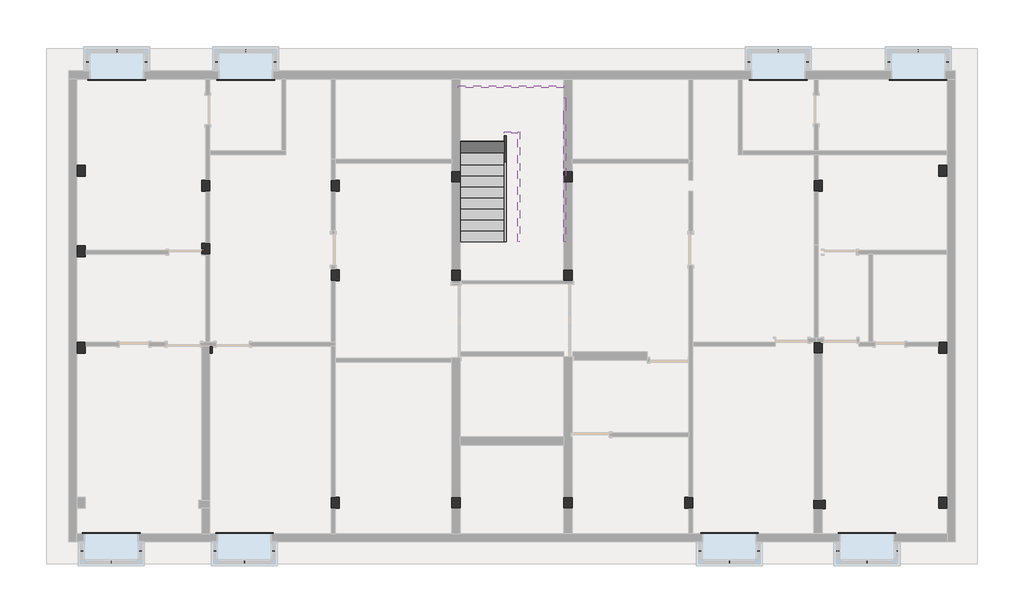
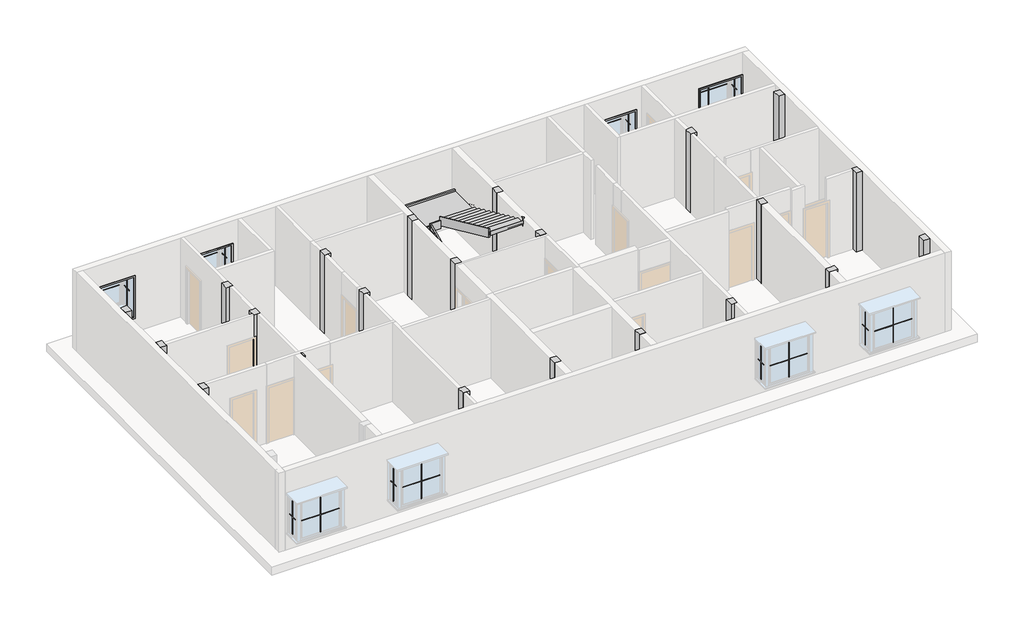
# One storey, part 3 of 3: 32 proxies, 22 columns, 6 members, 1 stair flight.
"""IFC4 building model written with IfcOpenShell, lengths in millimetres."""

from ifc_helpers import new_model, si_unit, frame, origin, place, context, project, spatial, polyline, outline, extrude, faceted_brep, transform, mapped, element, save
from components import m_muntin_pattern_2x2_m_muntin_pattern_2x2_c1fd4460, m_muntin_pattern_2x2_m_muntin_pattern_2x2_777b163a, m_trim_window_interior_flat_picture_frame_44e8afef, stair_flight_7b3ce822

model = new_model("IFC4")

# Units and contexts
model_context = context("Model", 3, world=origin())
ifc_project = project(units=[si_unit("LENGTHUNIT", "METRE", prefix="MILLI")], contexts=[model_context])

# Site, building, storey
site = spatial("IfcSite", under=ifc_project)
building = spatial("IfcBuilding", under=site)
storey = spatial("IfcBuildingStorey", under=building, Elevation=12801.6)

# Proxies
placement = place(None, origin())
m_muntin_pattern_2x2_m_muntin_pattern_2x2_shape = m_muntin_pattern_2x2_m_muntin_pattern_2x2_c1fd4460(model_context)
element("IfcBuildingElementProxy", 1, Name="M_Muntin Pattern_2x2 : M_Muntin Pattern_2x2", ObjectType="M_Muntin Pattern_2x2 : M_Muntin Pattern_2x2", at=placement, inside=storey, context=model_context, shape_type="MappedRepresentation", body=[
    mapped(m_muntin_pattern_2x2_m_muntin_pattern_2x2_shape, transform((-11500.7987957, -5499.9182661, 13522.25), x_axis=(-1.0, 0.0, 0.0), y_axis=(0.0, -1.0, 0.0), z_axis=(0.0, 0.0, 1.0))),
])
element("IfcBuildingElementProxy", 2, Name="M_Muntin Pattern_2x2 : M_Muntin Pattern_2x2", ObjectType="M_Muntin Pattern_2x2 : M_Muntin Pattern_2x2", at=placement, inside=storey, context=model_context, shape_type="MappedRepresentation", body=[
    mapped(m_muntin_pattern_2x2_m_muntin_pattern_2x2_shape, transform((-7819.250543, -5499.9182661, 13522.25), x_axis=(-1.0, 0.0, 0.0), y_axis=(0.0, -1.0, 0.0), z_axis=(0.0, 0.0, 1.0))),
])
element("IfcBuildingElementProxy", 3, Name="M_Muntin Pattern_2x2 : M_Muntin Pattern_2x2", ObjectType="M_Muntin Pattern_2x2 : M_Muntin Pattern_2x2", at=placement, inside=storey, context=model_context, shape_type="MappedRepresentation", body=[
    mapped(m_muntin_pattern_2x2_m_muntin_pattern_2x2_shape, transform((5599.7512082, -5499.9182661, 13522.25), x_axis=(-1.0, 0.0, 0.0), y_axis=(0.0, -1.0, 0.0), z_axis=(0.0, 0.0, 1.0))),
])
element("IfcBuildingElementProxy", 4, Name="M_Muntin Pattern_2x2 : M_Muntin Pattern_2x2", ObjectType="M_Muntin Pattern_2x2 : M_Muntin Pattern_2x2", at=placement, inside=storey, context=model_context, shape_type="MappedRepresentation", body=[
    mapped(m_muntin_pattern_2x2_m_muntin_pattern_2x2_shape, transform((9408.6146942, -5499.9182662, 13522.25), x_axis=(-1.0, 0.0, 0.0), y_axis=(0.0, -1.0, 0.0), z_axis=(0.0, 0.0, 1.0))),
])
element("IfcBuildingElementProxy", 5, Name="M_Muntin Pattern_2x2 : M_Muntin Pattern_2x2", ObjectType="M_Muntin Pattern_2x2 : M_Muntin Pattern_2x2", at=placement, inside=storey, context=model_context, shape_type="MappedRepresentation", body=[
    mapped(m_muntin_pattern_2x2_m_muntin_pattern_2x2_shape, transform((-11348.3987957, 8647.7317329, 13522.25), x_axis=(1.0, 0.0, 0.0), y_axis=(0.0, 1.0, 0.0), z_axis=(0.0, 0.0, 1.0))),
])
element("IfcBuildingElementProxy", 6, Name="M_Muntin Pattern_2x2 : M_Muntin Pattern_2x2", ObjectType="M_Muntin Pattern_2x2 : M_Muntin Pattern_2x2", at=placement, inside=storey, context=model_context, shape_type="MappedRepresentation", body=[
    mapped(m_muntin_pattern_2x2_m_muntin_pattern_2x2_shape, transform((-7779.6987993, 8647.7317329, 13522.25), x_axis=(1.0, 0.0, 0.0), y_axis=(0.0, 1.0, 0.0), z_axis=(0.0, 0.0, 1.0))),
])
element("IfcBuildingElementProxy", 7, Name="M_Muntin Pattern_2x2 : M_Muntin Pattern_2x2", ObjectType="M_Muntin Pattern_2x2 : M_Muntin Pattern_2x2", at=placement, inside=storey, context=model_context, shape_type="MappedRepresentation", body=[
    mapped(m_muntin_pattern_2x2_m_muntin_pattern_2x2_shape, transform((6952.301208, 8647.7317329, 13522.25), x_axis=(1.0, 0.0, 0.0), y_axis=(0.0, 1.0, 0.0), z_axis=(0.0, 0.0, 1.0))),
])
element("IfcBuildingElementProxy", 8, Name="M_Muntin Pattern_2x2 : M_Muntin Pattern_2x2", ObjectType="M_Muntin Pattern_2x2 : M_Muntin Pattern_2x2", at=placement, inside=storey, context=model_context, shape_type="MappedRepresentation", body=[
    mapped(m_muntin_pattern_2x2_m_muntin_pattern_2x2_shape, transform((10825.8012075, 8647.7317329, 13522.25), x_axis=(1.0, 0.0, 0.0), y_axis=(0.0, 1.0, 0.0), z_axis=(0.0, 0.0, 1.0))),
])
m_muntin_pattern_2x2_m_muntin_pattern_2x2_2_shape = m_muntin_pattern_2x2_m_muntin_pattern_2x2_777b163a(model_context)
element("IfcBuildingElementProxy", 9, Name="M_Muntin Pattern_2x2 : M_Muntin Pattern_2x2", ObjectType="M_Muntin Pattern_2x2 : M_Muntin Pattern_2x2", at=placement, inside=storey, context=model_context, shape_type="MappedRepresentation", body=[
    mapped(m_muntin_pattern_2x2_m_muntin_pattern_2x2_2_shape, transform((-10690.4737957, -5190.3932661, 13522.25), x_axis=(0.0, 1.0, 0.0), y_axis=(-1.0, 0.0, 0.0), z_axis=(0.0, 0.0, 1.0))),
])
element("IfcBuildingElementProxy", 10, Name="M_Muntin Pattern_2x2 : M_Muntin Pattern_2x2", ObjectType="M_Muntin Pattern_2x2 : M_Muntin Pattern_2x2", at=placement, inside=storey, context=model_context, shape_type="MappedRepresentation", body=[
    mapped(m_muntin_pattern_2x2_m_muntin_pattern_2x2_2_shape, transform((-12311.1237957, -5190.3932661, 13522.25), x_axis=(0.0, -1.0, 0.0), y_axis=(1.0, 0.0, 0.0), z_axis=(0.0, 0.0, 1.0))),
])
element("IfcBuildingElementProxy", 11, Name="M_Muntin Pattern_2x2 : M_Muntin Pattern_2x2", ObjectType="M_Muntin Pattern_2x2 : M_Muntin Pattern_2x2", at=placement, inside=storey, context=model_context, shape_type="MappedRepresentation", body=[
    mapped(m_muntin_pattern_2x2_m_muntin_pattern_2x2_2_shape, transform((-7008.925543, -5190.3932661, 13522.25), x_axis=(0.0, 1.0, 0.0), y_axis=(-1.0, 0.0, 0.0), z_axis=(0.0, 0.0, 1.0))),
])
element("IfcBuildingElementProxy", 12, Name="M_Muntin Pattern_2x2 : M_Muntin Pattern_2x2", ObjectType="M_Muntin Pattern_2x2 : M_Muntin Pattern_2x2", at=placement, inside=storey, context=model_context, shape_type="MappedRepresentation", body=[
    mapped(m_muntin_pattern_2x2_m_muntin_pattern_2x2_2_shape, transform((-8629.575543, -5190.3932661, 13522.25), x_axis=(0.0, -1.0, 0.0), y_axis=(1.0, 0.0, 0.0), z_axis=(0.0, 0.0, 1.0))),
])
element("IfcBuildingElementProxy", 13, Name="M_Muntin Pattern_2x2 : M_Muntin Pattern_2x2", ObjectType="M_Muntin Pattern_2x2 : M_Muntin Pattern_2x2", at=placement, inside=storey, context=model_context, shape_type="MappedRepresentation", body=[
    mapped(m_muntin_pattern_2x2_m_muntin_pattern_2x2_2_shape, transform((6410.0762082, -5190.3932661, 13522.25), x_axis=(0.0, 1.0, 0.0), y_axis=(-1.0, 0.0, 0.0), z_axis=(0.0, 0.0, 1.0))),
])
element("IfcBuildingElementProxy", 14, Name="M_Muntin Pattern_2x2 : M_Muntin Pattern_2x2", ObjectType="M_Muntin Pattern_2x2 : M_Muntin Pattern_2x2", at=placement, inside=storey, context=model_context, shape_type="MappedRepresentation", body=[
    mapped(m_muntin_pattern_2x2_m_muntin_pattern_2x2_2_shape, transform((4789.4262082, -5190.3932661, 13522.25), x_axis=(0.0, -1.0, 0.0), y_axis=(1.0, 0.0, 0.0), z_axis=(0.0, 0.0, 1.0))),
])
element("IfcBuildingElementProxy", 15, Name="M_Muntin Pattern_2x2 : M_Muntin Pattern_2x2", ObjectType="M_Muntin Pattern_2x2 : M_Muntin Pattern_2x2", at=placement, inside=storey, context=model_context, shape_type="MappedRepresentation", body=[
    mapped(m_muntin_pattern_2x2_m_muntin_pattern_2x2_2_shape, transform((10218.9396942, -5190.3932662, 13522.25), x_axis=(0.0, 1.0, 0.0), y_axis=(-1.0, 0.0, 0.0), z_axis=(0.0, 0.0, 1.0))),
])
element("IfcBuildingElementProxy", 16, Name="M_Muntin Pattern_2x2 : M_Muntin Pattern_2x2", ObjectType="M_Muntin Pattern_2x2 : M_Muntin Pattern_2x2", at=placement, inside=storey, context=model_context, shape_type="MappedRepresentation", body=[
    mapped(m_muntin_pattern_2x2_m_muntin_pattern_2x2_2_shape, transform((8598.2896942, -5190.3932661, 13522.25), x_axis=(0.0, -1.0, 0.0), y_axis=(1.0, 0.0, 0.0), z_axis=(0.0, 0.0, 1.0))),
])
element("IfcBuildingElementProxy", 17, Name="M_Muntin Pattern_2x2 : M_Muntin Pattern_2x2", ObjectType="M_Muntin Pattern_2x2 : M_Muntin Pattern_2x2", at=placement, inside=storey, context=model_context, shape_type="MappedRepresentation", body=[
    mapped(m_muntin_pattern_2x2_m_muntin_pattern_2x2_2_shape, transform((-12158.7237957, 8338.2067329, 13522.25), x_axis=(0.0, -1.0, 0.0), y_axis=(1.0, 0.0, 0.0), z_axis=(0.0, 0.0, 1.0))),
])
element("IfcBuildingElementProxy", 18, Name="M_Muntin Pattern_2x2 : M_Muntin Pattern_2x2", ObjectType="M_Muntin Pattern_2x2 : M_Muntin Pattern_2x2", at=placement, inside=storey, context=model_context, shape_type="MappedRepresentation", body=[
    mapped(m_muntin_pattern_2x2_m_muntin_pattern_2x2_2_shape, transform((-10538.0737957, 8338.2067329, 13522.25), x_axis=(0.0, 1.0, 0.0), y_axis=(-1.0, 0.0, 0.0), z_axis=(0.0, 0.0, 1.0))),
])
element("IfcBuildingElementProxy", 19, Name="M_Muntin Pattern_2x2 : M_Muntin Pattern_2x2", ObjectType="M_Muntin Pattern_2x2 : M_Muntin Pattern_2x2", at=placement, inside=storey, context=model_context, shape_type="MappedRepresentation", body=[
    mapped(m_muntin_pattern_2x2_m_muntin_pattern_2x2_2_shape, transform((-8590.0237993, 8338.2067329, 13522.25), x_axis=(0.0, -1.0, 0.0), y_axis=(1.0, 0.0, 0.0), z_axis=(0.0, 0.0, 1.0))),
])
element("IfcBuildingElementProxy", 20, Name="M_Muntin Pattern_2x2 : M_Muntin Pattern_2x2", ObjectType="M_Muntin Pattern_2x2 : M_Muntin Pattern_2x2", at=placement, inside=storey, context=model_context, shape_type="MappedRepresentation", body=[
    mapped(m_muntin_pattern_2x2_m_muntin_pattern_2x2_2_shape, transform((-6969.3737993, 8338.2067329, 13522.25), x_axis=(0.0, 1.0, 0.0), y_axis=(-1.0, 0.0, 0.0), z_axis=(0.0, 0.0, 1.0))),
])
element("IfcBuildingElementProxy", 21, Name="M_Muntin Pattern_2x2 : M_Muntin Pattern_2x2", ObjectType="M_Muntin Pattern_2x2 : M_Muntin Pattern_2x2", at=placement, inside=storey, context=model_context, shape_type="MappedRepresentation", body=[
    mapped(m_muntin_pattern_2x2_m_muntin_pattern_2x2_2_shape, transform((6141.976208, 8338.2067329, 13522.25), x_axis=(0.0, -1.0, 0.0), y_axis=(1.0, 0.0, 0.0), z_axis=(0.0, 0.0, 1.0))),
])
element("IfcBuildingElementProxy", 22, Name="M_Muntin Pattern_2x2 : M_Muntin Pattern_2x2", ObjectType="M_Muntin Pattern_2x2 : M_Muntin Pattern_2x2", at=placement, inside=storey, context=model_context, shape_type="MappedRepresentation", body=[
    mapped(m_muntin_pattern_2x2_m_muntin_pattern_2x2_2_shape, transform((7762.626208, 8338.2067329, 13522.25), x_axis=(0.0, 1.0, 0.0), y_axis=(-1.0, 0.0, 0.0), z_axis=(0.0, 0.0, 1.0))),
])
element("IfcBuildingElementProxy", 23, Name="M_Muntin Pattern_2x2 : M_Muntin Pattern_2x2", ObjectType="M_Muntin Pattern_2x2 : M_Muntin Pattern_2x2", at=placement, inside=storey, context=model_context, shape_type="MappedRepresentation", body=[
    mapped(m_muntin_pattern_2x2_m_muntin_pattern_2x2_2_shape, transform((10015.4762075, 8338.2067329, 13522.25), x_axis=(0.0, -1.0, 0.0), y_axis=(1.0, 0.0, 0.0), z_axis=(0.0, 0.0, 1.0))),
])
element("IfcBuildingElementProxy", 24, Name="M_Muntin Pattern_2x2 : M_Muntin Pattern_2x2", ObjectType="M_Muntin Pattern_2x2 : M_Muntin Pattern_2x2", at=placement, inside=storey, context=model_context, shape_type="MappedRepresentation", body=[
    mapped(m_muntin_pattern_2x2_m_muntin_pattern_2x2_2_shape, transform((11636.1262075, 8338.2067329, 13522.25), x_axis=(0.0, 1.0, 0.0), y_axis=(-1.0, 0.0, 0.0), z_axis=(0.0, 0.0, 1.0))),
])
m_trim_window_interior_flat_picture_frame_shape = m_trim_window_interior_flat_picture_frame_44e8afef(model_context)
element("IfcBuildingElementProxy", 25, Name="M_Trim-Window-Interior-Flat : Picture Frame", ObjectType="M_Trim-Window-Interior-Flat : Picture Frame", at=placement, inside=storey, context=model_context, shape_type="MappedRepresentation", body=[
    mapped(m_trim_window_interior_flat_picture_frame_shape, transform((-11500.7987957, -4712.5932661, 14952.4), x_axis=(-1.0, 0.0, 0.0), y_axis=(0.0, 0.0, 1.0), z_axis=(0.0, 1.0, 0.0))),
])
element("IfcBuildingElementProxy", 26, Name="M_Trim-Window-Interior-Flat : Picture Frame", ObjectType="M_Trim-Window-Interior-Flat : Picture Frame", at=placement, inside=storey, context=model_context, shape_type="MappedRepresentation", body=[
    mapped(m_trim_window_interior_flat_picture_frame_shape, transform((-7819.250543, -4712.5932661, 14952.4), x_axis=(-1.0, 0.0, 0.0), y_axis=(0.0, 0.0, 1.0), z_axis=(0.0, 1.0, 0.0))),
])
element("IfcBuildingElementProxy", 27, Name="M_Trim-Window-Interior-Flat : Picture Frame", ObjectType="M_Trim-Window-Interior-Flat : Picture Frame", at=placement, inside=storey, context=model_context, shape_type="MappedRepresentation", body=[
    mapped(m_trim_window_interior_flat_picture_frame_shape, transform((5599.7512082, -4712.5932661, 14952.4), x_axis=(-1.0, 0.0, 0.0), y_axis=(0.0, 0.0, 1.0), z_axis=(0.0, 1.0, 0.0))),
])
element("IfcBuildingElementProxy", 28, Name="M_Trim-Window-Interior-Flat : Picture Frame", ObjectType="M_Trim-Window-Interior-Flat : Picture Frame", at=placement, inside=storey, context=model_context, shape_type="MappedRepresentation", body=[
    mapped(m_trim_window_interior_flat_picture_frame_shape, transform((9408.6146942, -4712.5932661, 14952.4), x_axis=(-1.0, 0.0, 0.0), y_axis=(0.0, 0.0, 1.0), z_axis=(0.0, 1.0, 0.0))),
])
element("IfcBuildingElementProxy", 29, Name="M_Trim-Window-Interior-Flat : Picture Frame", ObjectType="M_Trim-Window-Interior-Flat : Picture Frame", at=placement, inside=storey, context=model_context, shape_type="MappedRepresentation", body=[
    mapped(m_trim_window_interior_flat_picture_frame_shape, transform((-11348.3987957, 7860.4067329, 14952.4), x_axis=(1.0, 0.0, 0.0), y_axis=(0.0, 0.0, 1.0), z_axis=(0.0, -1.0, 0.0))),
])
element("IfcBuildingElementProxy", 30, Name="M_Trim-Window-Interior-Flat : Picture Frame", ObjectType="M_Trim-Window-Interior-Flat : Picture Frame", at=placement, inside=storey, context=model_context, shape_type="MappedRepresentation", body=[
    mapped(m_trim_window_interior_flat_picture_frame_shape, transform((-7779.6987993, 7860.4067329, 14952.4), x_axis=(1.0, 0.0, 0.0), y_axis=(0.0, 0.0, 1.0), z_axis=(0.0, -1.0, 0.0))),
])
element("IfcBuildingElementProxy", 31, Name="M_Trim-Window-Interior-Flat : Picture Frame", ObjectType="M_Trim-Window-Interior-Flat : Picture Frame", at=placement, inside=storey, context=model_context, shape_type="MappedRepresentation", body=[
    mapped(m_trim_window_interior_flat_picture_frame_shape, transform((6952.301208, 7860.4067329, 14952.4), x_axis=(1.0, 0.0, 0.0), y_axis=(0.0, 0.0, 1.0), z_axis=(0.0, -1.0, 0.0))),
])
element("IfcBuildingElementProxy", 32, Name="M_Trim-Window-Interior-Flat : Picture Frame", ObjectType="M_Trim-Window-Interior-Flat : Picture Frame", at=placement, inside=storey, context=model_context, shape_type="MappedRepresentation", body=[
    mapped(m_trim_window_interior_flat_picture_frame_shape, transform((10825.8012075, 7860.4067329, 14952.4), x_axis=(1.0, 0.0, 0.0), y_axis=(0.0, 0.0, 1.0), z_axis=(0.0, -1.0, 0.0))),
])

# Columns
element("IfcColumn", 33, ObjectType="Rectangular Column : 1'X 9\"", at=placement, inside=storey, context=model_context, shape_type="SweptSolid", body=[
    extrude(outline(polyline([(-12224.6987957, 583.3067334), (-12224.6987957, 278.5067334), (-12453.2987957, 278.5067334), (-12453.2987957, 583.3067334), (-12224.6987957, 583.3067334)])), frame((0.0, 0.0, 12801.6), z_axis=(0.0, 0.0, 1.0), x_axis=(1.0, 0.0, 0.0)), (0.0, 0.0, 1.0), 3048.0),
])
element("IfcColumn", 34, ObjectType="Rectangular Column : 1'X 9\"", at=placement, inside=storey, context=model_context, shape_type="SweptSolid", body=[
    extrude(outline(polyline([(-12224.6987957, 3256.6567332), (-12224.6987957, 2951.8567332), (-12453.2987957, 2951.8567332), (-12453.2987957, 3256.6567332), (-12224.6987957, 3256.6567332)])), frame((0.0, 0.0, 12801.6), z_axis=(0.0, 0.0, 1.0), x_axis=(1.0, 0.0, 0.0)), (0.0, 0.0, 1.0), 3048.0),
])
element("IfcColumn", 35, ObjectType="Rectangular Column : 1'X 9\"", at=placement, inside=storey, context=model_context, shape_type="Brep", body=[
    faceted_brep([(-8770.2987992, 5066.406733, 12801.6), (-8770.2987992, 4761.606733, 12801.6), (-8884.5987992, 4761.606733, 12801.6), (-8998.8987992, 4761.606733, 12801.6), (-8998.8987992, 5066.406733, 12801.6), (-8884.5987992, 5066.406733, 12801.6), (-8770.2987992, 5066.406733, 15849.6), (-8770.2987992, 4761.606733, 15849.6), (-8884.5987992, 4761.606733, 15849.6), (-8998.8987992, 4761.606733, 15849.6), (-8998.8987992, 5066.406733, 15849.6), (-8884.5987992, 5066.406733, 15849.6)], [[[0, 1, 2, 3, 4, 5]], [[6, 7, 1, 0]], [[7, 8, 9, 3, 2, 1]], [[9, 10, 4, 3]], [[10, 11, 6, 0, 5, 4]], [[6, 11, 10, 9, 8, 7]]]),
])
element("IfcColumn", 36, ObjectType="Rectangular Column : 1'X 9\"", at=placement, inside=storey, context=model_context, shape_type="Brep", body=[
    faceted_brep([(-8770.2987992, 3326.5067332, 12801.6), (-8770.2987992, 3021.7067332, 12801.6), (-8884.598796, 3021.7067332, 12801.6), (-8998.8987992, 3021.7067332, 12801.6), (-8998.8987992, 3326.5067332, 12801.6), (-8884.5987992, 3326.5067332, 12801.6), (-8770.2987992, 3326.5067332, 15849.6), (-8770.2987992, 3021.7067332, 15849.6), (-8884.598796, 3021.7067332, 15849.6), (-8998.8987992, 3021.7067332, 15849.6), (-8998.8987992, 3326.5067332, 15849.6), (-8884.5987992, 3326.5067332, 15849.6)], [[[0, 1, 2, 3, 4, 5]], [[6, 7, 1, 0]], [[7, 8, 9, 3, 2, 1]], [[9, 10, 4, 3]], [[10, 11, 6, 0, 5, 4]], [[6, 11, 10, 9, 8, 7]]]),
])
element("IfcColumn", 37, ObjectType="Rectangular Column : 1'X 9\"", at=placement, inside=storey, context=model_context, shape_type="SweptSolid", body=[
    extrude(outline(polyline([(-8713.148796, 278.5067334), (-8771.750543, 278.5067334), (-8771.750543, 469.0067334), (-8713.148796, 469.0067334), (-8713.148796, 278.5067334)])), frame((0.0, 0.0, 12801.6), z_axis=(0.0, 0.0, 1.0), x_axis=(1.0, 0.0, 0.0)), (0.0, 0.0, 1.0), 3048.0),
])
element("IfcColumn", 38, ObjectType="Rectangular Column : 1'X 9\"", at=placement, inside=storey, context=model_context, shape_type="Brep", body=[
    faceted_brep([(-5188.8987995, 5066.406733, 12801.6), (-5188.8987995, 4761.606733, 12801.6), (-5303.1987995, 4761.606733, 12801.6), (-5417.4987995, 4761.606733, 12801.6), (-5417.4987995, 5066.406733, 12801.6), (-5303.1987995, 5066.406733, 12801.6), (-5188.8987995, 5066.406733, 15849.6), (-5188.8987995, 4761.606733, 15849.6), (-5303.1987995, 4761.606733, 15849.6), (-5417.4987995, 4761.606733, 15849.6), (-5417.4987995, 5066.406733, 15849.6), (-5303.1987995, 5066.406733, 15849.6)], [[[0, 1, 2, 3, 4, 5]], [[6, 7, 1, 0]], [[7, 8, 9, 3, 2, 1]], [[9, 10, 4, 3]], [[10, 11, 6, 0, 5, 4]], [[6, 11, 10, 9, 8, 7]]]),
])
element("IfcColumn", 39, ObjectType="Rectangular Column : 1'X 9\"", at=placement, inside=storey, context=model_context, shape_type="Brep", body=[
    faceted_brep([(-5188.8987995, 2589.9067802, 12801.6), (-5188.8987995, 2285.1067802, 12801.6), (-5303.1987995, 2285.1067802, 12801.6), (-5417.4987995, 2285.1067802, 12801.6), (-5417.4987995, 2589.9067802, 12801.6), (-5303.1987995, 2589.9067802, 12801.6), (-5188.8987995, 2589.9067802, 15849.6), (-5188.8987995, 2285.1067802, 15849.6), (-5303.1987995, 2285.1067802, 15849.6), (-5417.4987995, 2285.1067802, 15849.6), (-5417.4987995, 2589.9067802, 15849.6), (-5303.1987995, 2589.9067802, 15849.6)], [[[0, 1, 2, 3, 4, 5]], [[6, 7, 1, 0]], [[7, 8, 9, 3, 2, 1]], [[9, 10, 4, 3]], [[10, 11, 6, 0, 5, 4]], [[6, 11, 10, 9, 8, 7]]]),
])
element("IfcColumn", 40, ObjectType="Rectangular Column : 1'X 9\"", at=placement, inside=storey, context=model_context, shape_type="Brep", body=[
    faceted_brep([(-5188.8987963, -3709.2932193, 12801.6), (-5188.8987963, -4014.0932193, 12801.6), (-5303.1987963, -4014.0932193, 12801.6), (-5417.4987963, -4014.0932193, 12801.6), (-5417.4987963, -3709.2932193, 12801.6), (-5303.1987995, -3709.2932193, 12801.6), (-5188.8987963, -3709.2932193, 15849.6), (-5188.8987963, -4014.0932193, 15849.6), (-5303.1987963, -4014.0932193, 15849.6), (-5417.4987963, -4014.0932193, 15849.6), (-5417.4987963, -3709.2932193, 15849.6), (-5303.1987995, -3709.2932193, 15849.6)], [[[0, 1, 2, 3, 4, 5]], [[6, 7, 1, 0]], [[7, 8, 9, 3, 2, 1]], [[9, 10, 4, 3]], [[10, 11, 6, 0, 5, 4]], [[6, 11, 10, 9, 8, 7]]]),
])
element("IfcColumn", 41, ObjectType="Rectangular Column : 1'X 9\"", at=placement, inside=storey, context=model_context, shape_type="SweptSolid", body=[
    extrude(outline(polyline([(1250.0012085, -3709.2932193), (1250.0012085, -4014.0932193), (1021.4012085, -4014.0932193), (1021.4012085, -3709.2932193), (1250.0012085, -3709.2932193)])), frame((0.0, 0.0, 12801.6), z_axis=(0.0, 0.0, 1.0), x_axis=(1.0, 0.0, 0.0)), (0.0, 0.0, 1.0), 3048.0),
])
element("IfcColumn", 42, ObjectType="Rectangular Column : 1'X 9\"", at=placement, inside=storey, context=model_context, shape_type="Brep", body=[
    faceted_brep([(4590.1012082, -3709.2932193, 12801.6), (4590.1012082, -4014.0932193, 12801.6), (4475.8012082, -4014.0932193, 12801.6), (4361.5012082, -4014.0932193, 12801.6), (4361.5012082, -3709.2932193, 12801.6), (4475.8012082, -3709.2932193, 12801.6), (4590.1012082, -3709.2932193, 15849.6), (4590.1012082, -4014.0932193, 15849.6), (4475.8012082, -4014.0932193, 15849.6), (4361.5012082, -4014.0932193, 15849.6), (4361.5012082, -3709.2932193, 15849.6), (4475.8012082, -3709.2932193, 15849.6)], [[[0, 1, 2, 3, 4, 5]], [[6, 7, 1, 0]], [[7, 8, 9, 3, 2, 1]], [[9, 10, 4, 3]], [[10, 11, 6, 0, 5, 4]], [[6, 11, 10, 9, 8, 7]]]),
])
element("IfcColumn", 43, ObjectType="Rectangular Column : 1'X 9\"", at=placement, inside=storey, context=model_context, shape_type="SweptSolid", body=[
    extrude(outline(polyline([(11625.9012075, -3709.2932671), (11625.9012075, -4014.0932671), (11397.3012075, -4014.0932671), (11397.3012075, -3709.2932671), (11625.9012075, -3709.2932671)])), frame((0.0, 0.0, 12801.6), z_axis=(0.0, 0.0, 1.0), x_axis=(1.0, 0.0, 0.0)), (0.0, 0.0, 1.0), 3048.0),
])
element("IfcColumn", 44, ObjectType="Rectangular Column : 1'X 9\"", at=placement, inside=storey, context=model_context, shape_type="Brep", body=[
    faceted_brep([(11625.9012075, 583.3067295, 12801.6), (11625.9012075, 278.5067295, 12801.6), (11397.3012075, 278.5067295, 12801.6), (11397.3012075, 469.0067295, 12801.6), (11397.3012075, 583.3067295, 12801.6), (11625.9012075, 583.3067295, 15849.6), (11625.9012075, 278.5067295, 15849.6), (11397.3012075, 278.5067295, 15849.6), (11397.3012075, 469.0067295, 15849.6), (11397.3012075, 583.3067295, 15849.6)], [[[0, 1, 2, 3, 4]], [[5, 6, 1, 0]], [[6, 7, 2, 1]], [[7, 8, 9, 4, 3, 2]], [[9, 5, 0, 4]], [[5, 9, 8, 7, 6]]]),
])
element("IfcColumn", 45, ObjectType="Rectangular Column : 1'X 9\"", at=placement, inside=storey, context=model_context, shape_type="SweptSolid", body=[
    extrude(outline(polyline([(11625.9012075, 5479.1567329), (11625.9012075, 5174.3567329), (11397.3012075, 5174.3567329), (11397.3012075, 5479.1567329), (11625.9012075, 5479.1567329)])), frame((0.0, 0.0, 12801.6), z_axis=(0.0, 0.0, 1.0), x_axis=(1.0, 0.0, 0.0)), (0.0, 0.0, 1.0), 3048.0),
])
element("IfcColumn", 46, ObjectType="Rectangular Column : 1'X 9\"", at=placement, inside=storey, context=model_context, shape_type="Brep", body=[
    faceted_brep([(8172.5040565, 5065.4824989, 12801.6), (8172.5040565, 4760.6824989, 12801.6), (8057.2012047, 4760.6824989, 12801.6), (7943.9040565, 4760.6824989, 12801.6), (7943.9040565, 5065.4824989, 12801.6), (8058.2040565, 5065.4824989, 12801.6), (8172.5040565, 5065.4824989, 15849.6), (8172.5040565, 4760.6824989, 15849.6), (8057.2012047, 4760.6824989, 15849.6), (7943.9040565, 4760.6824989, 15849.6), (7943.9040565, 5065.4824989, 15849.6), (8058.2040565, 5065.4824989, 15849.6)], [[[0, 1, 2, 3, 4, 5]], [[6, 7, 1, 0]], [[7, 8, 9, 3, 2, 1]], [[9, 10, 4, 3]], [[10, 11, 6, 0, 5, 4]], [[6, 11, 10, 9, 8, 7]]]),
])
element("IfcColumn", 47, ObjectType="Rectangular Column : 1'X 9\"", at=placement, inside=storey, context=model_context, shape_type="Brep", body=[
    faceted_brep([(8171.5012047, 583.3067334, 12801.6), (8171.5012047, 278.5067334, 12801.6), (7942.9012047, 278.5067334, 12801.6), (7942.9012047, 583.3067334, 12801.6), (8000.0512079, 583.3067334, 12801.6), (8171.5012047, 583.3067334, 15849.6), (8171.5012047, 278.5067334, 15849.6), (7942.9012047, 278.5067334, 15849.6), (7942.9012047, 583.3067334, 15849.6), (8000.0512079, 583.3067334, 15849.6)], [[[0, 1, 2, 3, 4]], [[5, 6, 1, 0]], [[6, 7, 2, 1]], [[7, 8, 3, 2]], [[8, 9, 5, 0, 4, 3]], [[5, 9, 8, 7, 6]]]),
])
element("IfcColumn", 48, ObjectType="Rectangular Column : 1'X 9\"", at=placement, inside=storey, context=model_context, shape_type="Brep", body=[
    faceted_brep([(7941.7646942, -3787.3914801, 12801.6), (8246.5646942, -3787.3914801, 12801.6), (8246.5646942, -4015.9914801, 12801.6), (8170.3646942, -4015.9914801, 12801.6), (7941.7646942, -4015.9914801, 12801.6), (7941.7646942, -3787.3914801, 15849.6), (8246.5646942, -3787.3914801, 15849.6), (8246.5646942, -4015.9914801, 15849.6), (8170.3646942, -4015.9914801, 15849.6), (7941.7646942, -4015.9914801, 15849.6)], [[[0, 1, 2, 3, 4]], [[5, 6, 1, 0]], [[6, 7, 2, 1]], [[7, 8, 9, 4, 3, 2]], [[9, 5, 0, 4]], [[5, 9, 8, 7, 6]]]),
])
element("IfcColumn", 49, ObjectType="Rectangular Column : 1'X 9\"", at=placement, inside=storey, context=model_context, shape_type="SweptSolid", body=[
    extrude(outline(polyline([(-12453.2987957, 5174.3567339), (-12453.2987957, 5479.1567339), (-12224.6987957, 5479.1567339), (-12224.6987957, 5174.3567339), (-12453.2987957, 5174.3567339)])), frame((0.0, 0.0, 12801.6), z_axis=(0.0, 0.0, 1.0), x_axis=(1.0, 0.0, 0.0)), (0.0, 0.0, 1.0), 3048.0),
])
element("IfcColumn", 50, ObjectType="Rectangular Column : 1'X 9\"", at=placement, inside=storey, context=model_context, shape_type="SweptSolid", body=[
    extrude(outline(polyline([(-1845.5417538, 5320.4067329), (-1845.5417538, 5015.6067329), (-2074.1417538, 5015.6067329), (-2074.1417538, 5320.4067329), (-1845.5417538, 5320.4067329)])), frame((0.0, 0.0, 12801.6), z_axis=(0.0, 0.0, 1.0), x_axis=(1.0, 0.0, 0.0)), (0.0, 0.0, 1.0), 3048.0),
])
element("IfcColumn", 51, ObjectType="Rectangular Column : 1'X 9\"", at=placement, inside=storey, context=model_context, shape_type="SweptSolid", body=[
    extrude(outline(polyline([(1250.0012085, 5320.4067329), (1250.0012085, 5015.6067329), (1021.4012085, 5015.6067329), (1021.4012085, 5320.4067329), (1250.0012085, 5320.4067329)])), frame((0.0, 0.0, 12801.6), z_axis=(0.0, 0.0, 1.0), x_axis=(1.0, 0.0, 0.0)), (0.0, 0.0, 1.0), 3048.0),
])
element("IfcColumn", 52, ObjectType="Rectangular Column : 1'X 9\"", at=placement, inside=storey, context=model_context, shape_type="SweptSolid", body=[
    extrude(outline(polyline([(-1845.5417538, 2589.906774), (-1845.5417538, 2285.106774), (-2074.1417538, 2285.106774), (-2074.1417538, 2589.906774), (-1845.5417538, 2589.906774)])), frame((0.0, 0.0, 12801.6), z_axis=(0.0, 0.0, 1.0), x_axis=(1.0, 0.0, 0.0)), (0.0, 0.0, 1.0), 3048.0),
])
element("IfcColumn", 53, ObjectType="Rectangular Column : 1'X 9\"", at=placement, inside=storey, context=model_context, shape_type="Brep", body=[
    faceted_brep([(1253.2582462, 2589.9067742, 12801.6), (1253.2582462, 2285.1067742, 12801.6), (1024.6582462, 2285.1067742, 12801.6), (1024.6582462, 2589.9067742, 12801.6), (1250.0012085, 2589.9067742, 12801.6), (1253.2582462, 2589.9067742, 15849.6), (1253.2582462, 2285.1067742, 15849.6), (1024.6582462, 2285.1067742, 15849.6), (1024.6582462, 2589.9067742, 15849.6), (1250.0012085, 2589.9067742, 15849.6)], [[[0, 1, 2, 3, 4]], [[5, 6, 1, 0]], [[6, 7, 2, 1]], [[7, 8, 3, 2]], [[8, 9, 5, 0, 4, 3]], [[5, 9, 8, 7, 6]]]),
])
element("IfcColumn", 54, ObjectType="Rectangular Column : 1'X 9\"", at=placement, inside=storey, context=model_context, shape_type="SweptSolid", body=[
    extrude(outline(polyline([(-1848.7987998, -3709.2932663), (-1848.7987998, -4014.0932663), (-2077.3987998, -4014.0932663), (-2077.3987998, -3709.2932663), (-1848.7987998, -3709.2932663)])), frame((0.0, 0.0, 12801.6), z_axis=(0.0, 0.0, 1.0), x_axis=(1.0, 0.0, 0.0)), (0.0, 0.0, 1.0), 3048.0),
])

# Members
element("IfcMember", 55, ObjectType="Stringer - 2\" Width", at=placement, inside=storey, context=model_context, shape_type="SweptSolid", body=[
    extrude(outline(polyline([(3364.6067329, 12801.6), (3364.6067329, 13001.4262721), (6445.4289342, 14401.8), (7182.0114168, 14401.8), (3661.5714168, 12801.6), (3364.6067329, 12801.6)])), frame((-1896.3417538, 0.0, 0.0), z_axis=(1.0, 0.0, 0.0), x_axis=(0.0, 1.0, 0.0)), (0.0, 0.0, 1.0), 50.8),
])
element("IfcMember", 56, ObjectType="Stringer - 2\" Width", at=placement, inside=storey, context=model_context, shape_type="SweptSolid", body=[
    extrude(outline(polyline([(-1896.3417538, 7631.8067329), (-1896.3417538, 7682.6067329), (1021.4012085, 7682.6067329), (1021.4012085, 7631.8067329), (-1896.3417538, 7631.8067329)])), frame((0.0, 0.0, 14097.0), z_axis=(0.0, 0.0, 1.0), x_axis=(1.0, 0.0, 0.0)), (0.0, 0.0, 1.0), 304.8),
])
element("IfcMember", 57, ObjectType="Stringer - 2\" Width", at=placement, inside=storey, context=model_context, shape_type="SweptSolid", body=[
    extrude(outline(polyline([(6618.562049, 14097.0), (3364.6067329, 15576.0705982), (3364.6067329, 15910.8808176), (7355.1445316, 14097.0), (6618.562049, 14097.0)])), frame((1021.4012085, 0.0, 0.0), z_axis=(1.0, 0.0, 0.0), x_axis=(0.0, 1.0, 0.0)), (0.0, 0.0, 1.0), 50.8),
])
element("IfcMember", 58, ObjectType="Stringer - 2\" Width", at=placement, inside=storey, context=model_context, shape_type="SweptSolid", body=[
    extrude(outline(polyline([(3364.6067329, 12801.6), (3364.6067329, 13001.4262721), (6361.8067329, 14363.7899085), (6361.8067329, 14028.9796892), (3661.5714168, 12801.6), (3364.6067329, 12801.6)])), frame((-629.5987998, 0.0, 0.0), z_axis=(1.0, 0.0, 0.0), x_axis=(0.0, 1.0, 0.0)), (0.0, 0.0, 1.0), 50.8),
])
element("IfcMember", 59, ObjectType="Stringer - 2\" Width", at=placement, inside=storey, context=model_context, shape_type="SweptSolid", body=[
    extrude(outline(polyline([(-629.5987998, 6361.8067329), (-629.5987998, 6412.6067329), (-248.5987915, 6412.6067329), (-248.5987915, 6361.8067329), (-629.5987998, 6361.8067329)])), frame((0.0, 0.0, 14097.0), z_axis=(0.0, 0.0, 1.0), x_axis=(1.0, 0.0, 0.0)), (0.0, 0.0, 1.0), 304.8),
])
element("IfcMember", 60, ObjectType="Stringer - 2\" Width", at=placement, inside=storey, context=model_context, shape_type="SweptSolid", body=[
    extrude(outline(polyline([(6412.6067329, 14525.4262721), (6412.6067329, 14190.6160528), (3364.6067329, 15576.0705982), (3364.6067329, 15910.8808176), (6412.6067329, 14525.4262721)])), frame((-248.5987915, 0.0, 0.0), z_axis=(1.0, 0.0, 0.0), x_axis=(0.0, 1.0, 0.0)), (0.0, 0.0, 1.0), 50.8),
])

# Stair flight
stair_flight_shape = stair_flight_7b3ce822(model_context)
element("IfcStairFlight", 61, ObjectType="2\" Tread 1\" Nosing 1/4\" Riser", at=placement, inside=storey, context=model_context, shape_type="MappedRepresentation", body=[
    mapped(stair_flight_shape, transform((0.0, 0.0, 0.0), x_axis=(1.0, 0.0, 0.0), y_axis=(0.0, 1.0, 0.0), z_axis=(0.0, 0.0, 1.0))),
])

save(model, "model.ifc")

# Revit data of these elements
# Type "M_Muntin Pattern_2x2 : M_Muntin Pattern_2x2"
#   Width [instance default] = 3' - 11.24409"
#   Thickness = 0' - 0 1/2"
#   Height [instance default] = 3' - 11.24409"
#   Distance = 0' - 0 3/4"
#   Interior Material [instance default] = none
#   Exterior Material [instance default] = none
#   Default Elevation = 0
# Type "M_Trim-Window-Interior-Flat : Picture Frame"
#   Trim Thickness_Picture Frame = 0' - 1.1811"
#   Trim Width = 0' - 2.3622"
#   Trim Thickness_with Sill = 0' - 0.7874"
#   Sill Thickness = 0' - 1.1811"
#   Opening Width [instance default] = 1' - 11.62205"
#   Opening Height [instance default] = 2' - 11.43307"
#   Default Elevation = 3' - 11.24409"
#   Sill = no
#   Picture Frame = yes
#   Trim Material [instance default] = none
# Type "Rectangular Column : 1'X 9\""
#   Assembly Code = "B1010200"
#   Depth = 1' - 0"
#   Offset Base = 0' - 0"
#   Offset Top = 0' - 0"
#   Width = 0' - 9"
#   Material = none
# Elements 1, 2, 3, 4, 5, 6, 7, 8 (IfcBuildingElementProxy, "M_Muntin Pattern_2x2 : M_Muntin Pattern_2x2")
#   Width = 4' - 5.55512"
#   Height = 4' - 5.55512"
#   Interior Material = Wood - Stained
#   Exterior Material = Clad - White
#   Phase Created = New Construction
#   Materials on its faces: "Clad - White", "Wood - Stained"
# Elements 9, 10, 11, 12, 13, 14, 15, 16, 17, 18, 19, 20, 21, 22, 23, 24 (IfcBuildingElementProxy, "M_Muntin Pattern_2x2 : M_Muntin Pattern_2x2")
#   Width = 1' - 2.12205"
#   Height = 4' - 5.55512"
#   Interior Material = Wood - Stained
#   Exterior Material = Clad - White
#   Phase Created = New Construction
#   Materials on its faces: "Clad - White", "Wood - Stained"
# Elements 25, 26, 27, 28, 29, 30, 31, 32 (IfcBuildingElementProxy, "M_Trim-Window-Interior-Flat : Picture Frame")
#   Opening Width = 4' - 11.05512"
#   Opening Height = 5' - 1.05512"
#   Trim Material = Wood - Stained
#   Phase Created = New Construction
#   Materials on its faces: "Wood - Stained"
# Elements 33, 34, 35, 36, 37, 38, 39, 40, 41, 42, 43, 44, 45, 46, 47, 48, 49, 50, 51, 52, 53, 54 (IfcColumn, "Rectangular Column : 1'X 9\"")
#   Phase Created = New Construction
#   Materials on its faces: "Default Wall"
# Elements 55, 56, 57, 58, 59, 60 (IfcMember, "Stringer - 2\" Width")
#   Phase Created = New Construction
# Element 61 (IfcStairFlight, "2\" Tread 1\" Nosing 1/4\" Riser")
#   Phase Created = New Construction
# Materials
#   "Clad - White": class "Wood", colour RGB 242 242 238, transparency 0, Cost = 0
#   "Wood - Stained": class "Wood", colour RGB 224 178 126, transparency 0, Cost = 0
#   "Default Wall": colour RGB 128 128 128, transparency 0, Cost = 0
